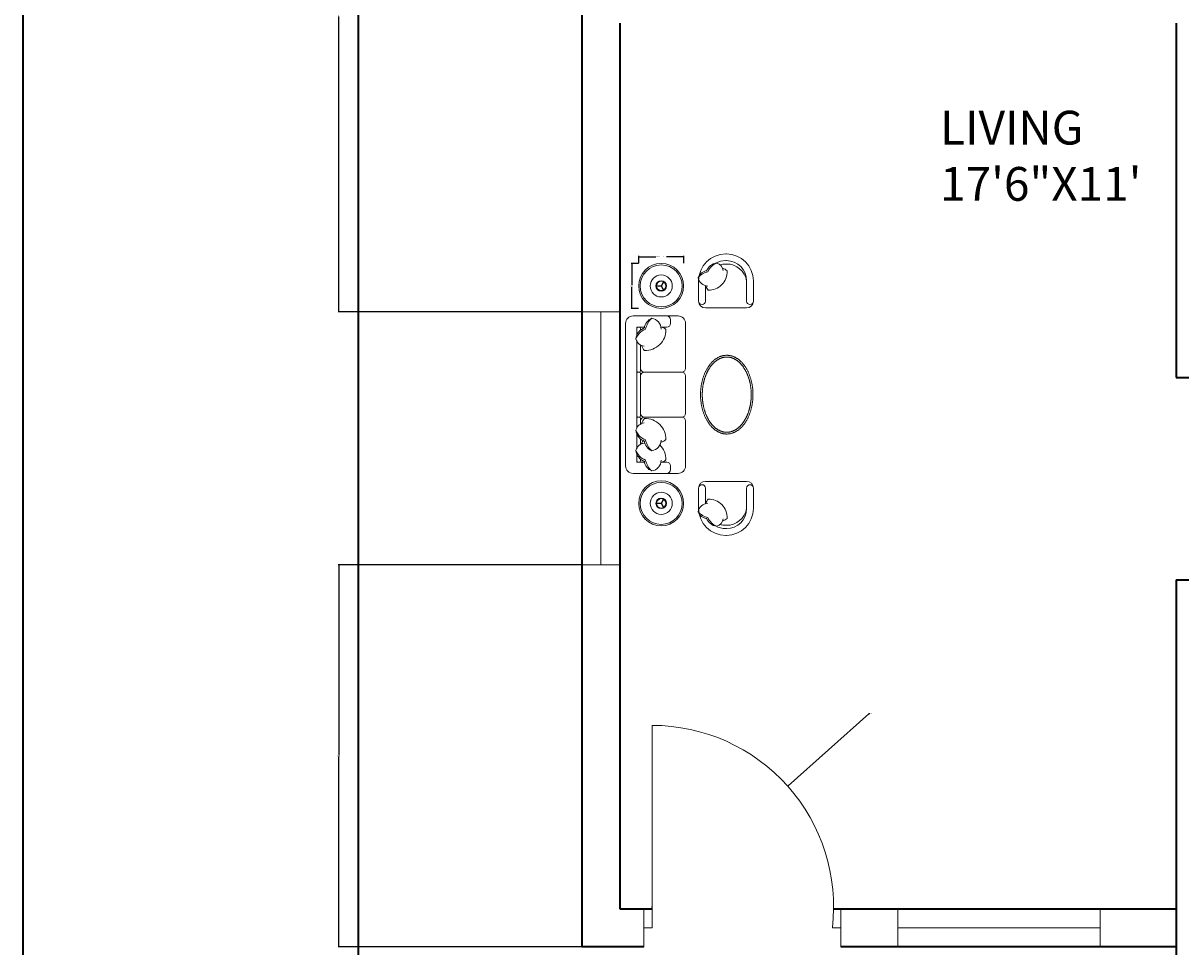
# Model space of a CAD drawing. Units: inches. Extents: x 1976 to 2558, y -977 to 2909.
# Tile 4 of 8: x 1976 to 2251, y 2026 to 2245. Entities that reach past the tile are written whole.
import ezdxf

# ---------------------------------------------------------------- set-up
doc = ezdxf.new("R2010")
doc.units = ezdxf.units.IN
for name, color, linetype, lineweight in [('A-ANNO-DIMS', 2, 'Continuous', 18), ('A-ANNO-TTLB', 7, 'Continuous', 35), ('A-AREA-IDEN', 7, 'Continuous', 18), ('A-DOOR', 3, 'Continuous', 18), ('A-FURN', 8, 'Continuous', 13), ('A-GLAZ', 4, 'Continuous', 18), ('A-WALL', 7, 'Continuous', 35)]:
    doc.layers.add(name, color=color, linetype=linetype, lineweight=lineweight)
doc.styles.get("Standard").update_dxf_attribs({"font": 'arial.ttf'})
doc.dimstyles.get("Standard").update_dxf_attribs({"dimtxt": 0.18, "dimasz": 0.18, "dimexe": 0.18, "dimexo": 0.0625, "dimgap": 0.09, "dimtad": 0, "dimtih": 1, "dimtoh": 1, "dimdec": 4, "dimzin": 0, "dimdsep": 46, "dimtxsty": 'Standard', "dimcen": 0.09, "dimadec": 0, "dimazin": 0, "dimtfac": 1, "dimtdec": 4, "dimtofl": 0, "dimtmove": 0, "dimatfit": 3, "dimfxl": 1, "dimtolj": 1, "dimtzin": 0, "dimarcsym": 0})

# ---------------------------------------------------------------- blocks, each defined once
blk = doc.blocks.new('TABLE-END-ROUND')
at = {"ltscale": 0.03}
for p, q in [((5.29, 5.36), (5.91, 6.45)), ((5.38, 5.31), (6.01, 6.39)), ((5.33, 5.39), (4.08, 5.39)), ((5.33, 5.28), (4.08, 5.28)), ((5.29, 5.31), (5.91, 4.22)), ((5.38, 5.36), (6.01, 4.28))]:
    blk.add_line(p, q, dxfattribs=at)
for radius in [5.33, 2.62, 1.25, 1.12]:
    blk.add_circle((5.33, 5.33), radius, dxfattribs=at)
blk.add_circle((5.33, 5.33), 4.98)
blk = doc.blocks.new('WIN-60-PLAN')
for p, q in [((4.5, 60), (0, 60)), ((0, 60), (9, 60)), ((4.5, 0), (4.5, 60)), ((0, 0), (9, 0)), ((9, 0), (4.5, 0))]:
    blk.add_line(p, q)
blk = doc.blocks.new('*D17')
at = {"layer": 'A-ANNO-DIMS', "color": 0, "lineweight": -2, "transparency": 16777216}
for p, q in [((2121.92, 2188.58), (2121.92, 2190.29)), ((2122.1, 2190.11), (2126, 2190.11)), ((2132.41, 2190.11), (2128.51, 2190.11)), ((2132.59, 2188.58), (2132.59, 2190.29))]:
    blk.add_line(p, q, dxfattribs=at)
at = {"layer": 'A-ANNO-DIMS', "color": 0, "transparency": 16777216}
for points in [[(2122.1, 2190.14), (2122.1, 2190.08), (2121.92, 2190.11)], [(2132.41, 2190.14), (2132.41, 2190.08), (2132.59, 2190.11)]]:
    blk.add_solid(points, dxfattribs=at)
at = {"layer": 'Defpoints', "color": 0, "transparency": 16777216}
for p in [(2132.59, 2190.11), (2121.92, 2188.51), (2132.59, 2188.51)]:
    blk.add_point(p, dxfattribs=at)
at = {"layer": 'A-ANNO-DIMS', "color": 0, "transparency": 16777216, "insert": (2127.26, 2190.11), "char_height": 0.18, "attachment_point": 5}
blk.add_mtext('\\A1;END TABLE 11 TYP.', dxfattribs=at)
blk = doc.blocks.new('*D18')
at = {"layer": 'A-ANNO-DIMS', "color": 0, "lineweight": -2, "transparency": 16777216}
for p, q in [((2121.86, 2188.51), (2120.14, 2188.51)), ((2120.32, 2188.33), (2120.32, 2183.36)), ((2120.32, 2178.03), (2120.32, 2183)), ((2121.86, 2177.85), (2120.14, 2177.85))]:
    blk.add_line(p, q, dxfattribs=at)
at = {"layer": 'A-ANNO-DIMS', "color": 0, "transparency": 16777216}
for points in [[(2120.29, 2188.33), (2120.35, 2188.33), (2120.32, 2188.51)], [(2120.29, 2178.03), (2120.35, 2178.03), (2120.32, 2177.85)]]:
    blk.add_solid(points, dxfattribs=at)
at = {"layer": 'Defpoints', "color": 0, "transparency": 16777216}
for p in [(2120.32, 2188.51), (2121.92, 2188.51), (2121.92, 2177.85)]:
    blk.add_point(p, dxfattribs=at)
at = {"layer": 'A-ANNO-DIMS', "color": 0, "transparency": 16777216, "insert": (2120.32, 2183.18), "char_height": 0.18, "attachment_point": 5}
blk.add_mtext('\\A1;11 TYP.', dxfattribs=at)
blk = doc.blocks.new('*D35')
at = {"layer": 'A-ANNO-DIMS', "color": 0, "lineweight": -2, "transparency": 16777216}
for p, q in [((2108.38, 2317.5), (2050.58, 2317.5)), ((2050.76, 2317.32), (2050.76, 2247.46)), ((2050.76, 2177.24), (2050.76, 2247.1)), ((2108.38, 2177.06), (2050.58, 2177.06))]:
    blk.add_line(p, q, dxfattribs=at)
at = {"layer": 'A-ANNO-DIMS', "color": 0, "transparency": 16777216}
for points in [[(2050.73, 2317.32), (2050.79, 2317.32), (2050.76, 2317.5)], [(2050.73, 2177.24), (2050.79, 2177.24), (2050.76, 2177.06)]]:
    blk.add_solid(points, dxfattribs=at)
at = {"layer": 'Defpoints', "color": 0, "transparency": 16777216}
for p in [(2108.44, 2317.5), (2050.76, 2177.06), (2108.44, 2177.06)]:
    blk.add_point(p, dxfattribs=at)
at = {"layer": 'A-ANNO-DIMS', "color": 0, "transparency": 16777216, "insert": (2050.76, 2247.28), "char_height": 0.18, "attachment_point": 5}
blk.add_mtext('\\A1;140.44', dxfattribs=at)
blk = doc.blocks.new('*D36')
at = {"layer": 'A-ANNO-DIMS', "color": 0, "lineweight": -2, "transparency": 16777216}
for p, q in [((2108.38, 2117.06), (2050.58, 2117.06)), ((2050.76, 2116.88), (2050.76, 2071.95)), ((2050.76, 2026.66), (2050.76, 2071.59)), ((2108.38, 2026.48), (2050.58, 2026.48))]:
    blk.add_line(p, q, dxfattribs=at)
at = {"layer": 'A-ANNO-DIMS', "color": 0, "transparency": 16777216}
for points in [[(2050.73, 2116.88), (2050.79, 2116.88), (2050.76, 2117.06)], [(2050.73, 2026.66), (2050.79, 2026.66), (2050.76, 2026.48)]]:
    blk.add_solid(points, dxfattribs=at)
at = {"layer": 'Defpoints', "color": 0, "transparency": 16777216}
for p in [(2108.44, 2117.06), (2050.76, 2026.48), (2108.44, 2026.48)]:
    blk.add_point(p, dxfattribs=at)
at = {"layer": 'A-ANNO-DIMS', "color": 0, "transparency": 16777216, "insert": (2050.76, 2071.77), "char_height": 0.18, "attachment_point": 5}
blk.add_mtext('\\A1;90.58', dxfattribs=at)
blk = doc.blocks.new('*D88')
at = {"layer": 'A-ANNO-DIMS', "color": 0, "lineweight": -2, "transparency": 16777216}
for p, q in [((2176.55, 2081.75), (2157.4, 2064.69)), ((2176.73, 2081.75), (2176.55, 2081.75)), ((2125.03, 2035.93), (2125.21, 2035.93)), ((2125.12, 2035.84), (2125.12, 2036.02))]:
    blk.add_line(p, q, dxfattribs=at)
at = {"layer": 'A-ANNO-DIMS', "color": 0, "transparency": 16777216}
blk.add_solid([(2157.38, 2064.71), (2157.42, 2064.66), (2157.27, 2064.57)], dxfattribs=at)
at = {"layer": 'Defpoints', "color": 0, "transparency": 16777216}
for p in [(2157.27, 2064.57), (2125.12, 2035.93)]:
    blk.add_point(p, dxfattribs=at)
at = {"layer": 'A-ANNO-DIMS', "color": 0, "transparency": 16777216, "insert": (2177.21, 2081.75), "char_height": 0.18, "attachment_point": 5}
blk.add_mtext('\\A1;R43.05', dxfattribs=at)

msp = doc.modelspace()

# ---------------------------------------------------------------- linework, layer by layer
at = {"layer": 'A-ANNO-TTLB'}
for points in [[(1975.8545, 2909.3429), (2557.9168, 2909.3429), (2557.9168, 1747.8598), (1975.8545, 1747.8598)], [(2055.4343, 2428.9091), (2450.0007, 2428.9091), (2450.0007, 1815.3916), (2055.4343, 1815.3916)]]:
    msp.add_lwpolyline(points, close=True, dxfattribs=at)
at = {"layer": 'A-DOOR'}
for p, q in [((2125.1248, 2030.9789), (2125.1248, 2078.9789)), ((2123.1248, 2035.4789), (2123.1248, 2026.4789)), ((2169.8866, 2035.4789), (2169.8866, 2026.4789)), ((2123.1248, 2026.4789), (2123.1248, 2030.9789)), ((2123.1248, 2030.9789), (2125.1248, 2030.9789)), ((2169.8866, 2030.9789), (2167.8866, 2030.9789)), ((2169.8866, 2026.4789), (2169.8866, 2030.9789))]:
    msp.add_line(p, q, dxfattribs=at)
msp.add_arc((2125.1248, 2035.9313), 43.0476, 353.393764, 90, dxfattribs=at)
at = {"layer": 'A-FURN', "ltscale": 0.03}
for points in [[(2142.6352, 2177.9535), (2147.5242, 2177.9535, 0.41421356), (2149.1272, 2179.5565), (2149.1272, 2184.3654, 0.41421356), (2142.7153, 2190.7772), (2142.6352, 2190.7772), (2142.555, 2190.7772, 0.41421356), (2136.1432, 2184.3654), (2136.1432, 2179.5565, 0.41421356), (2137.7462, 2177.9535), (2142.6352, 2177.9535)], [(2142.6352, 2136.8478), (2147.5242, 2136.8478, -0.41421356), (2149.1272, 2135.2449), (2149.1272, 2130.436, -0.41421356), (2142.7153, 2124.0241), (2142.6352, 2124.0241), (2142.555, 2124.0241, -0.41421356), (2136.1432, 2130.436), (2136.1432, 2135.2449, -0.41421356), (2137.7462, 2136.8478), (2142.6352, 2136.8478)]]:
    msp.add_lwpolyline(points, format="xyb", dxfattribs=at)
at = {"layer": 'A-FURN'}
for points in [[(2136.0121, 2185.1744, -0.14772988), (2138.3546, 2186.5519, -0.21334276), (2140.4215, 2188.5721, -0.17866181)], [(2138.3087, 2183.1542, -0.35677236), (2136.0121, 2185.1744, -0.24954205), (2138.093, 2186.8393, 9.61688035)], [(2137.9047, 2183.2031, 0.16554063), (2138.4005, 2182.1441, 0.42598917), (2142.9018, 2186.7355, 0.12152332), (2141.8333, 2187.3684, -7.11546429)], [(2138.031, 2186.6616, -0.30666349), (2140.4215, 2188.5721, -0.30632997), (2141.9832, 2186.8273, 0.87284716)], [(2140.168, 2188.54, -0.13059149), (2142.555, 2189.1743), (2142.6352, 2189.1743)], [(2141.1886, 2188.2001, -0.07238424), (2142.555, 2188.3728), (2142.6352, 2188.3728)], [(2147.5242, 2184.3654, 0.41421356), (2142.7153, 2189.1743), (2142.6352, 2189.1743)], [(2147.5242, 2184.3654, 0.37271891), (2142.7153, 2188.3728), (2142.6352, 2188.3728)], [(2147.5242, 2184.3654), (2147.5242, 2179.5565, 0.41421356), (2148.3257, 2178.755), (2148.3257, 2178.755, 0.41421356), (2149.1272, 2179.5565)], [(2137.7462, 2183.2416), (2137.7462, 2179.5565, -0.41421356), (2136.9447, 2178.755), (2136.9447, 2178.755, -0.41421356), (2136.1432, 2179.5565)], [(2128.5903, 2176.0679, -0.41421356), (2129.4793, 2175.179), (2129.4793, 2174.2901, -0.41421356), (2128.5903, 2173.4012), (2127.2131, 2173.4012)], [(2125.0263, 2175.5022, 0.14772988), (2123.4986, 2172.9041, 0.21334276), (2121.258, 2170.6117, 0.17866181)], [(2123.3768, 2173.263, 0.30666349), (2121.258, 2170.6117, 0.30632997), (2123.193, 2168.8797, -0.87284716)], [(2122.3679, 2172.7228), (2122.3679, 2173.0456, 0.41421356), (2122.0124, 2173.4012), (2121.8346, 2173.4012, 0.41421356), (2121.479, 2173.0456)], [(2121.479, 2173.0456), (2121.479, 2171.5311, 0.41421356)], [(2127.2127, 2173.4031, -0.16554063), (2128.3872, 2172.8532, -0.42598917), (2123.2949, 2167.8609, -0.12152332), (2122.593, 2169.0459, 7.11546429)], [(2127.2669, 2172.9551, 0.35677236), (2125.0263, 2175.5022, 0.24954205), (2123.1798, 2173.1943, -9.61688035)], [(2121.479, 2170.0523), (2121.479, 2163.0897, 0.41421356), (2121.8346, 2162.7342), (2122.0124, 2162.7342, 0.41421356), (2122.3679, 2163.0897), (2122.3679, 2169.1572, 0.41421356)], [(2122.3679, 2163.6231, 0.41421356), (2123.2568, 2162.7342), (2132.146, 2162.7342, 0.41421356)], [(2122.3679, 2161.8453, -0.41421356), (2123.2568, 2162.7342)], [(2121.479, 2149.5376), (2121.479, 2151.7116, -0.41421356), (2121.8346, 2152.0672), (2122.0124, 2152.0672, -0.41421356), (2122.3679, 2151.7116), (2122.3679, 2150.4327, -0.41421356)], [(2122.3679, 2152.9561, 0.41421356), (2123.2568, 2152.0672)], [(2122.3679, 2151.1783, -0.41421356), (2123.2568, 2152.0672), (2132.146, 2152.0672, -0.41421356)], [(2127.2127, 2146.1868, 0.16554063), (2128.3872, 2146.7367, 0.42598917), (2123.2949, 2151.7291, 0.12152332), (2122.593, 2150.544, -7.11546429)], [(2123.3768, 2146.3269, -0.30666349), (2121.258, 2148.9782, -0.30632997), (2123.193, 2150.7102, 0.87284716)], [(2125.0263, 2144.0878, -0.14772988), (2123.4986, 2146.6858, -0.21334276), (2121.258, 2148.9782, -0.17866181)], [(2123.3768, 2141.5383, -0.30666349), (2121.258, 2144.1896, -0.30632997), (2123.193, 2145.9217, 0.87284716)], [(2121.479, 2144.7491), (2121.479, 2148.0588, -0.41421356)], [(2122.3679, 2146.8671), (2122.3679, 2145.6442, -0.41421356)], [(2122.9405, 2146.5007, 0.07186538), (2122.593, 2145.7554, -7.11546429)], [(2127.2669, 2146.6349, -0.35677236), (2125.0263, 2144.0878, -0.24954205), (2123.1798, 2146.3957, 9.61688035)], [(2125.0263, 2139.2992, -0.14772988), (2123.4986, 2141.8972, -0.21334276), (2121.258, 2144.1896, -0.17866181)], [(2121.479, 2143.2702), (2121.479, 2141.4002), (2123.2259, 2141.4002, -0.41421356)], [(2121.479, 2141.7558), (2121.479, 2143.2702, -0.41421356)], [(2127.2127, 2141.3983, 0.16554063), (2128.3872, 2141.9482, 0.20023115), (2126.9568, 2145.4769, 0.12152332)], [(2122.3679, 2142.0786), (2122.3679, 2141.7558, -0.41421356), (2122.0124, 2141.4002), (2121.8346, 2141.4002, -0.41421356), (2121.479, 2141.7558)], [(2127.2669, 2141.8463, -0.35677236), (2125.0263, 2139.2992, -0.24954205), (2123.1798, 2141.6071, 9.61688035)], [(2127.2131, 2141.4002), (2128.5903, 2141.4002, -0.41421356), (2129.4793, 2140.5113), (2129.4793, 2139.6224, -0.41421356), (2128.5903, 2138.7335)], [(2137.7462, 2131.5597), (2137.7462, 2135.2449, 0.41421356), (2136.9447, 2136.0464), (2136.9447, 2136.0464, 0.41421356), (2136.1432, 2135.2449)], [(2147.5242, 2130.4359), (2147.5242, 2135.2449, -0.41421356), (2148.3257, 2136.0464), (2148.3257, 2136.0464, -0.41421356), (2149.1272, 2135.2449)], [(2137.9047, 2131.5983, -0.16554063), (2138.4005, 2132.6573, -0.42598917), (2142.9018, 2128.0658, -0.12152332), (2141.8333, 2127.433, 7.11546429)], [(2138.3087, 2131.6472, 0.35677236), (2136.0121, 2129.6269, 0.24954205), (2138.093, 2127.9621, -9.61688035)], [(2136.0121, 2129.6269, 0.14772988), (2138.3546, 2128.2495, 0.21334276), (2140.4215, 2126.2293, 0.17866181)], [(2147.5242, 2130.436, -0.37271891), (2142.7153, 2126.4286), (2142.6352, 2126.4286)], [(2147.5242, 2130.436, -0.41421356), (2142.7153, 2125.6271), (2142.6352, 2125.6271)], [(2138.031, 2128.1397, 0.30666349), (2140.4215, 2126.2293, 0.30632997), (2141.9832, 2127.974, -0.87284716)], [(2140.168, 2126.2614, 0.13059149), (2142.555, 2125.6271), (2142.6352, 2125.6271)], [(2141.1886, 2126.6013, 0.07238424), (2142.555, 2126.4286), (2142.6352, 2126.4286)]]:
    msp.add_lwpolyline(points, format="xyb", dxfattribs=at)
at = {"layer": 'A-FURN', "ltscale": 0.03}
msp.add_lwpolyline([(2131.2571, 2176.0679, -0.41421356), (2133.0349, 2174.2901), (2133.0349, 2163.6231, -0.41421356), (2132.146, 2162.7342, -0.41421356), (2133.0349, 2161.8453), (2133.0349, 2152.9561, -0.41421356), (2132.146, 2152.0672, -0.41421356), (2133.0349, 2151.1783), (2133.0349, 2140.5113, -0.41421356), (2131.2571, 2138.7335), (2120.5901, 2138.7335, -0.41421356), (2118.8123, 2140.5113), (2118.8123, 2174.2901, -0.41421356), (2120.5901, 2176.0679)], format="xyb", close=True, dxfattribs=at)
at = {"layer": 'A-FURN'}
for points in [[(2123.2259, 2173.4012), (2121.479, 2173.4012), (2121.479, 2171.5311)], [(2121.479, 2170.0523), (2121.479, 2149.5376)], [(2121.479, 2148.0588), (2121.479, 2144.7491)]]:
    msp.add_lwpolyline(points, dxfattribs=at)
msp.add_lwpolyline([(2121.479, 2152.4228), (2121.479, 2162.3786, -0.41421356), (2121.8346, 2162.7342), (2122.0124, 2162.7342, -0.41421356), (2122.3679, 2162.3786), (2122.3679, 2152.4228, -0.41421356), (2122.0124, 2152.0672), (2121.8346, 2152.0672, -0.41421356)], format="xyb", close=True, dxfattribs=at)
at = {"layer": 'A-FURN', "ltscale": 0.03}
msp.add_polyline3d([(2142.813, 2166.7343, 0), (2142.6952, 2166.7326, 0), (2142.5775, 2166.7276, 0), (2142.4599, 2166.7192, 0), (2142.3424, 2166.7076, 0), (2142.2251, 2166.6925, 0), (2142.1079, 2166.6742, 0), (2141.9911, 2166.6525, 0), (2141.8745, 2166.6275, 0), (2141.7583, 2166.5992, 0), (2141.6424, 2166.5676, 0), (2141.5269, 2166.5328, 0), (2141.412, 2166.4946, 0), (2141.2975, 2166.4532, 0), (2141.1836, 2166.4086, 0), (2141.0702, 2166.3607, 0), (2140.9575, 2166.3096, 0), (2140.8454, 2166.2554, 0), (2140.734, 2166.1979, 0), (2140.6234, 2166.1374, 0), (2140.5136, 2166.0736, 0), (2140.4046, 2166.0068, 0), (2140.2965, 2165.9369, 0), (2140.1892, 2165.8639, 0), (2140.0829, 2165.7879, 0), (2139.9776, 2165.709, 0), (2139.8733, 2165.627, 0), (2139.77, 2165.5421, 0), (2139.6678, 2165.4542, 0), (2139.5668, 2165.3635, 0), (2139.4669, 2165.2699, 0), (2139.3682, 2165.1735, 0), (2139.2708, 2165.0744, 0), (2139.1746, 2164.9724, 0), (2139.0797, 2164.8678, 0), (2138.9862, 2164.7605, 0), (2138.894, 2164.6505, 0), (2138.8033, 2164.538, 0), (2138.714, 2164.4229, 0), (2138.6261, 2164.3053, 0), (2138.5397, 2164.1852, 0), (2138.4549, 2164.0627, 0), (2138.3716, 2163.9378, 0), (2138.29, 2163.8105, 0), (2138.2099, 2163.681, 0), (2138.1315, 2163.5492, 0), (2138.0548, 2163.4152, 0), (2137.9797, 2163.2791, 0), (2137.9064, 2163.1408, 0), (2137.8349, 2163.0005, 0), (2137.7651, 2162.8582, 0), (2137.6972, 2162.7139, 0), (2137.6311, 2162.5678, 0), (2137.5668, 2162.4198, 0), (2137.5044, 2162.2699, 0), (2137.444, 2162.1184, 0), (2137.3854, 2161.9651, 0), (2137.3288, 2161.8102, 0), (2137.2741, 2161.6538, 0), (2137.2215, 2161.4958, 0), (2137.1708, 2161.3363, 0), (2137.1222, 2161.1755, 0), (2137.0756, 2161.0133, 0), (2137.031, 2160.8497, 0), (2136.9885, 2160.685, 0), (2136.9481, 2160.5191, 0), (2136.9098, 2160.352, 0), (2136.8737, 2160.1839, 0), (2136.8396, 2160.0148, 0), (2136.8077, 2159.8448, 0), (2136.7779, 2159.6739, 0), (2136.7503, 2159.5022, 0), (2136.7249, 2159.3297, 0), (2136.7017, 2159.1566, 0), (2136.6806, 2158.9828, 0), (2136.6618, 2158.8084, 0), (2136.6451, 2158.6336, 0), (2136.6306, 2158.4582, 0), (2136.6184, 2158.2826, 0), (2136.6084, 2158.1066, 0), (2136.6006, 2157.9303, 0), (2136.595, 2157.7539, 0), (2136.5917, 2157.5773, 0), (2136.5906, 2157.4007, 0), (2136.5917, 2157.224, 0), (2136.595, 2157.0475, 0), (2136.6006, 2156.871, 0), (2136.6084, 2156.6948, 0), (2136.6184, 2156.5188, 0), (2136.6306, 2156.3431, 0), (2136.6451, 2156.1678, 0), (2136.6618, 2155.9929, 0), (2136.6806, 2155.8186, 0), (2136.7017, 2155.6448, 0), (2136.7249, 2155.4716, 0), (2136.7503, 2155.2992, 0), (2136.7779, 2155.1274, 0), (2136.8077, 2154.9565, 0), (2136.8396, 2154.7865, 0), (2136.8737, 2154.6174, 0), (2136.9098, 2154.4493, 0), (2136.9481, 2154.2823, 0), (2136.9885, 2154.1164, 0), (2137.031, 2153.9516, 0), (2137.0756, 2153.7881, 0), (2137.1222, 2153.6259, 0), (2137.1708, 2153.465, 0), (2137.2215, 2153.3056, 0), (2137.2741, 2153.1476, 0), (2137.3288, 2152.9911, 0), (2137.3854, 2152.8362, 0), (2137.444, 2152.683, 0), (2137.5044, 2152.5314, 0), (2137.5668, 2152.3816, 0), (2137.6311, 2152.2336, 0), (2137.6972, 2152.0874, 0), (2137.7651, 2151.9431, 0), (2137.8349, 2151.8008, 0), (2137.9064, 2151.6605, 0), (2137.9797, 2151.5223, 0), (2138.0548, 2151.3861, 0), (2138.1315, 2151.2521, 0), (2138.2099, 2151.1204, 0), (2138.29, 2150.9908, 0), (2138.3716, 2150.8636, 0), (2138.4549, 2150.7387, 0), (2138.5397, 2150.6161, 0), (2138.6261, 2150.4961, 0), (2138.714, 2150.3785, 0), (2138.8033, 2150.2634, 0), (2138.894, 2150.1508, 0), (2138.9862, 2150.0409, 0), (2139.0797, 2149.9336, 0), (2139.1746, 2149.8289, 0), (2139.2708, 2149.727, 0), (2139.3682, 2149.6278, 0), (2139.4669, 2149.5314, 0), (2139.5668, 2149.4379, 0), (2139.6678, 2149.3471, 0), (2139.77, 2149.2593, 0), (2139.8733, 2149.1744, 0), (2139.9776, 2149.0924, 0), (2140.0829, 2149.0134, 0), (2140.1892, 2148.9374, 0), (2140.2965, 2148.8645, 0), (2140.4046, 2148.7945, 0), (2140.5136, 2148.7277, 0), (2140.6234, 2148.664, 0), (2140.734, 2148.6034, 0), (2140.8454, 2148.546, 0), (2140.9575, 2148.4917, 0), (2141.0702, 2148.4406, 0), (2141.1836, 2148.3928, 0), (2141.2975, 2148.3481, 0), (2141.412, 2148.3067, 0), (2141.5269, 2148.2686, 0), (2141.6424, 2148.2337, 0), (2141.7583, 2148.2021, 0), (2141.8745, 2148.1738, 0), (2141.9911, 2148.1489, 0), (2142.1079, 2148.1272, 0), (2142.2251, 2148.1088, 0), (2142.3424, 2148.0938, 0), (2142.4599, 2148.0821, 0), (2142.5775, 2148.0738, 0), (2142.6952, 2148.0687, 0), (2142.813, 2148.0671, 0), (2142.9307, 2148.0687, 0), (2143.0484, 2148.0738, 0), (2143.1661, 2148.0821, 0), (2143.2836, 2148.0938, 0), (2143.4009, 2148.1088, 0), (2143.518, 2148.1272, 0), (2143.6349, 2148.1489, 0), (2143.7515, 2148.1738, 0), (2143.8677, 2148.2021, 0), (2143.9836, 2148.2337, 0), (2144.099, 2148.2686, 0), (2144.214, 2148.3067, 0), (2144.3285, 2148.3481, 0), (2144.4424, 2148.3928, 0), (2144.5558, 2148.4406, 0), (2144.6685, 2148.4917, 0), (2144.7806, 2148.546, 0), (2144.8919, 2148.6034, 0), (2145.0025, 2148.664, 0), (2145.1124, 2148.7277, 0), (2145.2214, 2148.7945, 0), (2145.3295, 2148.8645, 0), (2145.4368, 2148.9374, 0), (2145.5431, 2149.0134, 0), (2145.6484, 2149.0924, 0), (2145.7527, 2149.1744, 0), (2145.8559, 2149.2593, 0), (2145.9581, 2149.3471, 0), (2146.0592, 2149.4379, 0), (2146.159, 2149.5314, 0), (2146.2577, 2149.6278, 0), (2146.3552, 2149.727, 0), (2146.4513, 2149.8289, 0), (2146.5462, 2149.9336, 0), (2146.6397, 2150.0409, 0), (2146.7319, 2150.1508, 0), (2146.8227, 2150.2634, 0), (2146.912, 2150.3785, 0), (2146.9999, 2150.4961, 0), (2147.0862, 2150.6161, 0), (2147.1711, 2150.7387, 0), (2147.2543, 2150.8636, 0), (2147.336, 2150.9908, 0), (2147.4161, 2151.1204, 0), (2147.4945, 2151.2521, 0), (2147.5712, 2151.3861, 0), (2147.6462, 2151.5223, 0), (2147.7195, 2151.6605, 0), (2147.7911, 2151.8008, 0), (2147.8608, 2151.9431, 0), (2147.9288, 2152.0874, 0), (2147.9949, 2152.2336, 0), (2148.0591, 2152.3816, 0), (2148.1215, 2152.5314, 0), (2148.182, 2152.683, 0), (2148.2406, 2152.8362, 0), (2148.2972, 2152.9911, 0), (2148.3518, 2153.1476, 0), (2148.4045, 2153.3056, 0), (2148.4552, 2153.465, 0), (2148.5038, 2153.6259, 0), (2148.5504, 2153.7881, 0), (2148.595, 2153.9516, 0), (2148.6374, 2154.1164, 0), (2148.6778, 2154.2823, 0), (2148.7161, 2154.4493, 0), (2148.7523, 2154.6174, 0), (2148.7863, 2154.7865, 0), (2148.8183, 2154.9565, 0), (2148.848, 2155.1274, 0), (2148.8756, 2155.2992, 0), (2148.901, 2155.4716, 0), (2148.9243, 2155.6448, 0), (2148.9453, 2155.8186, 0), (2148.9642, 2155.9929, 0), (2148.9809, 2156.1678, 0), (2148.9953, 2156.3431, 0), (2149.0075, 2156.5188, 0), (2149.0176, 2156.6948, 0), (2149.0254, 2156.871, 0), (2149.0309, 2157.0475, 0), (2149.0343, 2157.224, 0), (2149.0354, 2157.4007, 0), (2149.0343, 2157.5773, 0), (2149.0309, 2157.7539, 0), (2149.0254, 2157.9303, 0), (2149.0176, 2158.1066, 0), (2149.0075, 2158.2826, 0), (2148.9953, 2158.4582, 0), (2148.9809, 2158.6336, 0), (2148.9642, 2158.8084, 0), (2148.9453, 2158.9828, 0), (2148.9243, 2159.1566, 0), (2148.901, 2159.3297, 0), (2148.8756, 2159.5022, 0), (2148.848, 2159.6739, 0), (2148.8183, 2159.8448, 0), (2148.7863, 2160.0148, 0), (2148.7523, 2160.1839, 0), (2148.7161, 2160.352, 0), (2148.6778, 2160.5191, 0), (2148.6374, 2160.685, 0), (2148.595, 2160.8497, 0), (2148.5504, 2161.0133, 0), (2148.5038, 2161.1755, 0), (2148.4552, 2161.3363, 0), (2148.4045, 2161.4958, 0), (2148.3518, 2161.6538, 0), (2148.2972, 2161.8102, 0), (2148.2406, 2161.9651, 0), (2148.182, 2162.1184, 0), (2148.1215, 2162.2699, 0), (2148.0591, 2162.4198, 0), (2147.9949, 2162.5678, 0), (2147.9288, 2162.7139, 0), (2147.8608, 2162.8582, 0), (2147.7911, 2163.0005, 0), (2147.7195, 2163.1408, 0), (2147.6462, 2163.2791, 0), (2147.5712, 2163.4152, 0), (2147.4945, 2163.5492, 0), (2147.4161, 2163.681, 0), (2147.336, 2163.8105, 0), (2147.2543, 2163.9378, 0), (2147.1711, 2164.0627, 0), (2147.0862, 2164.1852, 0), (2146.9999, 2164.3053, 0), (2146.912, 2164.4229, 0), (2146.8227, 2164.538, 0), (2146.7319, 2164.6505, 0), (2146.6397, 2164.7605, 0), (2146.5462, 2164.8678, 0), (2146.4513, 2164.9724, 0), (2146.3552, 2165.0744, 0), (2146.2577, 2165.1735, 0), (2146.159, 2165.2699, 0), (2146.0592, 2165.3635, 0), (2145.9581, 2165.4542, 0), (2145.8559, 2165.5421, 0), (2145.7527, 2165.627, 0), (2145.6484, 2165.709, 0), (2145.5431, 2165.7879, 0), (2145.4368, 2165.8639, 0), (2145.3295, 2165.9369, 0), (2145.2214, 2166.0068, 0), (2145.1124, 2166.0736, 0), (2145.0025, 2166.1374, 0), (2144.8919, 2166.1979, 0), (2144.7806, 2166.2554, 0), (2144.6685, 2166.3096, 0), (2144.5558, 2166.3607, 0), (2144.4424, 2166.4086, 0), (2144.3285, 2166.4532, 0), (2144.214, 2166.4946, 0), (2144.099, 2166.5328, 0), (2143.9836, 2166.5676, 0), (2143.8677, 2166.5992, 0), (2143.7515, 2166.6275, 0), (2143.6349, 2166.6525, 0), (2143.518, 2166.6742, 0), (2143.4009, 2166.6925, 0), (2143.2836, 2166.7076, 0), (2143.1661, 2166.7192, 0), (2143.0484, 2166.7276, 0), (2142.9307, 2166.7326, 0), (2142.813, 2166.7343, 0)], dxfattribs=at)
at = {"layer": 'A-FURN'}
msp.add_polyline3d([(2142.813, 2166.3195, 0), (2142.7493, 2166.3189, 0), (2142.6854, 2166.3173, 0), (2142.6212, 2166.3145, 0), (2142.5567, 2166.3106, 0), (2142.4919, 2166.3056, 0), (2142.4269, 2166.2995, 0), (2142.3617, 2166.2921, 0), (2142.2962, 2166.2836, 0), (2142.2304, 2166.2739, 0), (2142.1645, 2166.2629, 0), (2142.0983, 2166.2508, 0), (2142.0319, 2166.2374, 0), (2141.9653, 2166.2227, 0), (2141.8986, 2166.2068, 0), (2141.8316, 2166.1896, 0), (2141.7645, 2166.1711, 0), (2141.6973, 2166.1513, 0), (2141.6298, 2166.1301, 0), (2141.5623, 2166.1077, 0), (2141.4946, 2166.0838, 0), (2141.4268, 2166.0586, 0), (2141.3588, 2166.032, 0), (2141.2908, 2166.004, 0), (2141.2227, 2165.9745, 0), (2141.1546, 2165.9437, 0), (2141.0865, 2165.9114, 0), (2141.0183, 2165.8778, 0), (2140.9502, 2165.8427, 0), (2140.8821, 2165.8062, 0), (2140.8141, 2165.7682, 0), (2140.7461, 2165.7289, 0), (2140.6783, 2165.6881, 0), (2140.6105, 2165.6459, 0), (2140.5429, 2165.6023, 0), (2140.4755, 2165.5572, 0), (2140.4083, 2165.5107, 0), (2140.3412, 2165.4627, 0), (2140.2744, 2165.4133, 0), (2140.2078, 2165.3625, 0), (2140.1414, 2165.3102, 0), (2140.0754, 2165.2565, 0), (2140.0096, 2165.2014, 0), (2139.9442, 2165.1446, 0), (2139.879, 2165.0864, 0), (2139.8143, 2165.0266, 0), (2139.7499, 2164.9653, 0), (2139.6859, 2164.9025, 0), (2139.6223, 2164.8383, 0), (2139.5591, 2164.7726, 0), (2139.4963, 2164.7055, 0), (2139.434, 2164.637, 0), (2139.3722, 2164.5671, 0), (2139.3108, 2164.4958, 0), (2139.25, 2164.4233, 0), (2139.1896, 2164.3494, 0), (2139.1299, 2164.2742, 0), (2139.0706, 2164.1978, 0), (2139.0119, 2164.1201, 0), (2138.9539, 2164.0412, 0), (2138.8964, 2163.9611, 0), (2138.8395, 2163.8799, 0), (2138.7833, 2163.7974, 0), (2138.7277, 2163.7138, 0), (2138.6729, 2163.6291, 0), (2138.6187, 2163.5434, 0), (2138.5652, 2163.4565, 0), (2138.5124, 2163.3686, 0), (2138.4604, 2163.2797, 0), (2138.4091, 2163.1897, 0), (2138.3586, 2163.0988, 0), (2138.3089, 2163.0069, 0), (2138.26, 2162.9141, 0), (2138.2119, 2162.8203, 0), (2138.1647, 2162.7257, 0), (2138.1183, 2162.6301, 0), (2138.0728, 2162.5338, 0), (2138.0282, 2162.4365, 0), (2137.9845, 2162.3385, 0), (2137.9418, 2162.2397, 0), (2137.9, 2162.1401, 0), (2137.8591, 2162.0398, 0), (2137.8193, 2161.9387, 0), (2137.7804, 2161.837, 0), (2137.7425, 2161.7347, 0), (2137.7056, 2161.6321, 0), (2137.6698, 2161.5292, 0), (2137.6349, 2161.4261, 0), (2137.601, 2161.3226, 0), (2137.5681, 2161.219, 0), (2137.5362, 2161.115, 0), (2137.5053, 2161.0109, 0), (2137.4754, 2160.9065, 0), (2137.4464, 2160.8018, 0), (2137.4184, 2160.697, 0), (2137.3913, 2160.5919, 0), (2137.3652, 2160.4866, 0), (2137.3401, 2160.3811, 0), (2137.3159, 2160.2754, 0), (2137.2926, 2160.1695, 0), (2137.2703, 2160.0635, 0), (2137.2489, 2159.9572, 0), (2137.2285, 2159.8508, 0), (2137.209, 2159.7443, 0), (2137.1904, 2159.6376, 0), (2137.1727, 2159.5307, 0), (2137.1559, 2159.4237, 0), (2137.1401, 2159.3166, 0), (2137.1251, 2159.2093, 0), (2137.1111, 2159.1019, 0), (2137.0979, 2158.9944, 0), (2137.0857, 2158.8868, 0), (2137.0743, 2158.7792, 0), (2137.0638, 2158.6714, 0), (2137.0542, 2158.5635, 0), (2137.0455, 2158.4556, 0), (2137.0376, 2158.3476, 0), (2137.0306, 2158.2395, 0), (2137.0245, 2158.1314, 0), (2137.0192, 2158.0232, 0), (2137.0148, 2157.915, 0), (2137.0113, 2157.8068, 0), (2137.0086, 2157.6985, 0), (2137.0067, 2157.5902, 0), (2137.0056, 2157.4819, 0), (2137.0054, 2157.3736, 0), (2137.006, 2157.2653, 0), (2137.0075, 2157.157, 0), (2137.0098, 2157.0487, 0), (2137.0129, 2156.9405, 0), (2137.0169, 2156.8322, 0), (2137.0218, 2156.724, 0), (2137.0275, 2156.6159, 0), (2137.034, 2156.5078, 0), (2137.0415, 2156.3998, 0), (2137.0497, 2156.2918, 0), (2137.0589, 2156.1839, 0), (2137.0689, 2156.0761, 0), (2137.0799, 2155.9683, 0), (2137.0917, 2155.8607, 0), (2137.1044, 2155.7532, 0), (2137.118, 2155.6457, 0), (2137.1325, 2155.5384, 0), (2137.1479, 2155.4312, 0), (2137.1642, 2155.3241, 0), (2137.1814, 2155.2172, 0), (2137.1995, 2155.1104, 0), (2137.2186, 2155.0038, 0), (2137.2386, 2154.8973, 0), (2137.2595, 2154.791, 0), (2137.2813, 2154.6848, 0), (2137.3041, 2154.5789, 0), (2137.3278, 2154.4731, 0), (2137.3525, 2154.3675, 0), (2137.3781, 2154.2621, 0), (2137.4047, 2154.1569, 0), (2137.4322, 2154.0519, 0), (2137.4607, 2153.9472, 0), (2137.4902, 2153.8427, 0), (2137.5207, 2153.7384, 0), (2137.5521, 2153.6343, 0), (2137.5845, 2153.5305, 0), (2137.6178, 2153.427, 0), (2137.6522, 2153.3237, 0), (2137.6876, 2153.2207, 0), (2137.7239, 2153.1179, 0), (2137.7613, 2153.0155, 0), (2137.7997, 2152.9134, 0), (2137.8391, 2152.812, 0), (2137.8794, 2152.7113, 0), (2137.9208, 2152.6113, 0), (2137.9631, 2152.5121, 0), (2138.0063, 2152.4137, 0), (2138.0504, 2152.3161, 0), (2138.0955, 2152.2193, 0), (2138.1414, 2152.1233, 0), (2138.1882, 2152.0283, 0), (2138.2358, 2151.9341, 0), (2138.2843, 2151.8408, 0), (2138.3336, 2151.7484, 0), (2138.3837, 2151.657, 0), (2138.4346, 2151.5665, 0), (2138.4863, 2151.4771, 0), (2138.5387, 2151.3887, 0), (2138.5918, 2151.3013, 0), (2138.6457, 2151.215, 0), (2138.7002, 2151.1297, 0), (2138.7554, 2151.0456, 0), (2138.8113, 2150.9626, 0), (2138.8679, 2150.8807, 0), (2138.925, 2150.8, 0), (2138.9828, 2150.7205, 0), (2139.0412, 2150.6422, 0), (2139.1002, 2150.5652, 0), (2139.1597, 2150.4894, 0), (2139.2197, 2150.4149, 0), (2139.2803, 2150.3416, 0), (2139.3414, 2150.2697, 0), (2139.403, 2150.1992, 0), (2139.4651, 2150.13, 0), (2139.5276, 2150.0622, 0), (2139.5906, 2149.9958, 0), (2139.654, 2149.9308, 0), (2139.7178, 2149.8673, 0), (2139.782, 2149.8052, 0), (2139.8466, 2149.7447, 0), (2139.9116, 2149.6857, 0), (2139.9768, 2149.6282, 0), (2140.0424, 2149.5722, 0), (2140.1083, 2149.5178, 0), (2140.1746, 2149.4648, 0), (2140.241, 2149.4132, 0), (2140.3077, 2149.3631, 0), (2140.3747, 2149.3145, 0), (2140.4419, 2149.2673, 0), (2140.5092, 2149.2215, 0), (2140.5767, 2149.1771, 0), (2140.6444, 2149.1342, 0), (2140.7122, 2149.0927, 0), (2140.7801, 2149.0526, 0), (2140.8481, 2149.014, 0), (2140.9162, 2148.9768, 0), (2140.9843, 2148.941, 0), (2141.0524, 2148.9066, 0), (2141.1206, 2148.8736, 0), (2141.1887, 2148.8421, 0), (2141.2568, 2148.8119, 0), (2141.3248, 2148.7832, 0), (2141.3928, 2148.7559, 0), (2141.4607, 2148.73, 0), (2141.5284, 2148.7055, 0), (2141.5961, 2148.6823, 0), (2141.6636, 2148.6605, 0), (2141.7309, 2148.64, 0), (2141.7981, 2148.6208, 0), (2141.8651, 2148.603, 0), (2141.932, 2148.5864, 0), (2141.9986, 2148.5711, 0), (2142.0651, 2148.5571, 0), (2142.1314, 2148.5443, 0), (2142.1975, 2148.5328, 0), (2142.2633, 2148.5225, 0), (2142.3289, 2148.5133, 0), (2142.3943, 2148.5054, 0), (2142.4595, 2148.4987, 0), (2142.5244, 2148.4931, 0), (2142.589, 2148.4886, 0), (2142.6533, 2148.4853, 0), (2142.7174, 2148.4831, 0), (2142.7812, 2148.482, 0), (2142.8448, 2148.482, 0), (2142.9085, 2148.4831, 0), (2142.9726, 2148.4853, 0), (2143.037, 2148.4886, 0), (2143.1016, 2148.4931, 0), (2143.1665, 2148.4987, 0), (2143.2316, 2148.5054, 0), (2143.297, 2148.5133, 0), (2143.3626, 2148.5225, 0), (2143.4285, 2148.5328, 0), (2143.4946, 2148.5443, 0), (2143.5608, 2148.5571, 0), (2143.6273, 2148.5711, 0), (2143.694, 2148.5864, 0), (2143.7608, 2148.603, 0), (2143.8279, 2148.6208, 0), (2143.8951, 2148.64, 0), (2143.9624, 2148.6605, 0), (2144.0299, 2148.6823, 0), (2144.0975, 2148.7055, 0), (2144.1653, 2148.73, 0), (2144.2332, 2148.7559, 0), (2144.3011, 2148.7832, 0), (2144.3692, 2148.8119, 0), (2144.4373, 2148.8421, 0), (2144.5054, 2148.8736, 0), (2144.5735, 2148.9066, 0), (2144.6417, 2148.941, 0), (2144.7098, 2148.9768, 0), (2144.7779, 2149.014, 0), (2144.8459, 2149.0526, 0), (2144.9138, 2149.0927, 0), (2144.9816, 2149.1342, 0), (2145.0492, 2149.1771, 0), (2145.1167, 2149.2215, 0), (2145.1841, 2149.2673, 0), (2145.2513, 2149.3145, 0), (2145.3182, 2149.3631, 0), (2145.3849, 2149.4132, 0), (2145.4514, 2149.4648, 0), (2145.5176, 2149.5178, 0), (2145.5835, 2149.5722, 0), (2145.6491, 2149.6282, 0), (2145.7144, 2149.6857, 0), (2145.7793, 2149.7447, 0), (2145.8439, 2149.8052, 0), (2145.9081, 2149.8673, 0), (2145.9719, 2149.9308, 0), (2146.0353, 2149.9958, 0), (2146.0983, 2150.0622, 0), (2146.1608, 2150.13, 0), (2146.2229, 2150.1992, 0), (2146.2845, 2150.2697, 0), (2146.3456, 2150.3416, 0), (2146.4062, 2150.4149, 0), (2146.4663, 2150.4894, 0), (2146.5258, 2150.5652, 0), (2146.5848, 2150.6422, 0), (2146.6431, 2150.7205, 0), (2146.7009, 2150.8, 0), (2146.7581, 2150.8807, 0), (2146.8146, 2150.9626, 0), (2146.8705, 2151.0456, 0), (2146.9257, 2151.1297, 0), (2146.9803, 2151.215, 0), (2147.0341, 2151.3013, 0), (2147.0873, 2151.3887, 0), (2147.1397, 2151.4771, 0), (2147.1913, 2151.5665, 0), (2147.2422, 2151.657, 0), (2147.2923, 2151.7484, 0), (2147.3416, 2151.8408, 0), (2147.3901, 2151.9341, 0), (2147.4378, 2152.0283, 0), (2147.4846, 2152.1233, 0), (2147.5305, 2152.2193, 0), (2147.5755, 2152.3161, 0), (2147.6197, 2152.4137, 0), (2147.6629, 2152.5121, 0), (2147.7052, 2152.6113, 0), (2147.7465, 2152.7113, 0), (2147.7869, 2152.812, 0), (2147.8263, 2152.9134, 0), (2147.8646, 2153.0155, 0), (2147.902, 2153.1179, 0), (2147.9384, 2153.2207, 0), (2147.9737, 2153.3237, 0), (2148.0081, 2153.427, 0), (2148.0415, 2153.5305, 0), (2148.0739, 2153.6343, 0), (2148.1053, 2153.7384, 0), (2148.1357, 2153.8427, 0), (2148.1652, 2153.9472, 0), (2148.1937, 2154.0519, 0), (2148.2212, 2154.1569, 0), (2148.2478, 2154.2621, 0), (2148.2734, 2154.3675, 0), (2148.2981, 2154.4731, 0), (2148.3218, 2154.5789, 0), (2148.3446, 2154.6848, 0), (2148.3665, 2154.791, 0), (2148.3874, 2154.8973, 0), (2148.4074, 2155.0038, 0), (2148.4264, 2155.1104, 0), (2148.4446, 2155.2172, 0), (2148.4618, 2155.3241, 0), (2148.4781, 2155.4312, 0), (2148.4935, 2155.5384, 0), (2148.508, 2155.6457, 0), (2148.5216, 2155.7532, 0), (2148.5343, 2155.8607, 0), (2148.5461, 2155.9683, 0), (2148.557, 2156.0761, 0), (2148.5671, 2156.1839, 0), (2148.5762, 2156.2918, 0), (2148.5845, 2156.3998, 0), (2148.5919, 2156.5078, 0), (2148.5985, 2156.6159, 0), (2148.6042, 2156.724, 0), (2148.609, 2156.8322, 0), (2148.613, 2156.9405, 0), (2148.6162, 2157.0487, 0), (2148.6184, 2157.157, 0), (2148.6199, 2157.2653, 0), (2148.6205, 2157.3736, 0), (2148.6203, 2157.4819, 0), (2148.6193, 2157.5902, 0), (2148.6174, 2157.6985, 0), (2148.6147, 2157.8068, 0), (2148.6111, 2157.915, 0), (2148.6067, 2158.0232, 0), (2148.6014, 2158.1314, 0), (2148.5953, 2158.2395, 0), (2148.5883, 2158.3476, 0), (2148.5805, 2158.4556, 0), (2148.5717, 2158.5635, 0), (2148.5621, 2158.6714, 0), (2148.5517, 2158.7792, 0), (2148.5403, 2158.8868, 0), (2148.528, 2158.9944, 0), (2148.5149, 2159.1019, 0), (2148.5008, 2159.2093, 0), (2148.4859, 2159.3166, 0), (2148.47, 2159.4237, 0), (2148.4533, 2159.5307, 0), (2148.4356, 2159.6376, 0), (2148.417, 2159.7443, 0), (2148.3975, 2159.8508, 0), (2148.377, 2159.9572, 0), (2148.3557, 2160.0635, 0), (2148.3334, 2160.1695, 0), (2148.3101, 2160.2754, 0), (2148.2859, 2160.3811, 0), (2148.2608, 2160.4866, 0), (2148.2347, 2160.5919, 0), (2148.2076, 2160.697, 0), (2148.1796, 2160.8018, 0), (2148.1506, 2160.9065, 0), (2148.1206, 2161.0109, 0), (2148.0897, 2161.115, 0), (2148.0578, 2161.219, 0), (2148.0249, 2161.3226, 0), (2147.991, 2161.4261, 0), (2147.9562, 2161.5292, 0), (2147.9203, 2161.6321, 0), (2147.8835, 2161.7347, 0), (2147.8456, 2161.837, 0), (2147.8067, 2161.9387, 0), (2147.7668, 2162.0398, 0), (2147.726, 2162.1401, 0), (2147.6842, 2162.2397, 0), (2147.6414, 2162.3385, 0), (2147.5977, 2162.4365, 0), (2147.5531, 2162.5338, 0), (2147.5076, 2162.6301, 0), (2147.4613, 2162.7257, 0), (2147.414, 2162.8203, 0), (2147.366, 2162.9141, 0), (2147.3171, 2163.0069, 0), (2147.2674, 2163.0988, 0), (2147.2169, 2163.1897, 0), (2147.1656, 2163.2797, 0), (2147.1136, 2163.3686, 0), (2147.0608, 2163.4565, 0), (2147.0073, 2163.5434, 0), (2146.9531, 2163.6291, 0), (2146.8982, 2163.7138, 0), (2146.8427, 2163.7974, 0), (2146.7864, 2163.8799, 0), (2146.7296, 2163.9611, 0), (2146.6721, 2164.0412, 0), (2146.614, 2164.1201, 0), (2146.5553, 2164.1978, 0), (2146.4961, 2164.2742, 0), (2146.4363, 2164.3494, 0), (2146.376, 2164.4233, 0), (2146.3151, 2164.4958, 0), (2146.2538, 2164.5671, 0), (2146.1919, 2164.637, 0), (2146.1296, 2164.7055, 0), (2146.0669, 2164.7726, 0), (2146.0037, 2164.8383, 0), (2145.9401, 2164.9025, 0), (2145.8761, 2164.9653, 0), (2145.8117, 2165.0266, 0), (2145.7469, 2165.0864, 0), (2145.6818, 2165.1446, 0), (2145.6164, 2165.2014, 0), (2145.5506, 2165.2565, 0), (2145.4845, 2165.3102, 0), (2145.4182, 2165.3625, 0), (2145.3516, 2165.4133, 0), (2145.2848, 2165.4627, 0), (2145.2177, 2165.5107, 0), (2145.1504, 2165.5572, 0), (2145.083, 2165.6023, 0), (2145.0154, 2165.6459, 0), (2144.9477, 2165.6881, 0), (2144.8798, 2165.7289, 0), (2144.8119, 2165.7682, 0), (2144.7438, 2165.8062, 0), (2144.6757, 2165.8427, 0), (2144.6076, 2165.8778, 0), (2144.5395, 2165.9114, 0), (2144.4713, 2165.9437, 0), (2144.4032, 2165.9745, 0), (2144.3351, 2166.004, 0), (2144.2671, 2166.032, 0), (2144.1992, 2166.0586, 0), (2144.1314, 2166.0838, 0), (2144.0637, 2166.1077, 0), (2143.9961, 2166.1301, 0), (2143.9287, 2166.1513, 0), (2143.8614, 2166.1711, 0), (2143.7943, 2166.1896, 0), (2143.7274, 2166.2068, 0), (2143.6606, 2166.2227, 0), (2143.5941, 2166.2374, 0), (2143.5277, 2166.2508, 0), (2143.4615, 2166.2629, 0), (2143.3955, 2166.2739, 0), (2143.3298, 2166.2836, 0), (2143.2643, 2166.2921, 0), (2143.199, 2166.2995, 0), (2143.134, 2166.3056, 0), (2143.0692, 2166.3106, 0), (2143.0048, 2166.3145, 0), (2142.9405, 2166.3173, 0), (2142.8766, 2166.3189, 0), (2142.813, 2166.3195, 0)], dxfattribs=at)
at = {"layer": 'A-GLAZ'}
for p, q in [((2183.4385, 2035.4789), (2183.4385, 2026.4789)), ((2231.4385, 2030.9789), (2231.4385, 2035.4789)), ((2231.4385, 2035.4789), (2231.4385, 2026.4789)), ((2183.4385, 2026.4789), (2183.4385, 2030.9789)), ((2183.4385, 2030.9789), (2231.4385, 2030.9789))]:
    msp.add_line(p, q, dxfattribs=at)
at = {"layer": 'A-WALL'}
for p, q in [((2108.4385, 2317.4977), (2108.4385, 2026.4789)), ((2117.4385, 2245.4789), (2117.4385, 2035.4789)), ((2117.4385, 2245.4789), (2117.4385, 2035.4789)), ((2249.4385, 2245.4789), (2249.4385, 2161.4789)), ((2249.4385, 2161.4789), (2260.6343, 2161.4789)), ((2249.4385, 2113.4789), (2260.6343, 2113.4789)), ((2249.4385, 2113.4789), (2249.4385, 1967.9789)), ((2117.4385, 2035.4789), (2125.1248, 2035.4789)), ((2168.17, 2035.4789), (2249.4385, 2035.4789)), ((2249.4385, 2035.4789), (2249.4385, 2026.4789)), ((2123.1248, 2026.4789), (2108.4385, 2026.4789)), ((2249.4385, 2026.4789), (2169.8866, 2026.4789))]:
    msp.add_line(p, q, dxfattribs=at)

# ---------------------------------------------------------------- block references
at = {"layer": 'A-FURN'}
msp.add_blockref('TABLE-END-ROUND', (2121.923, 2177.846), dxfattribs=at)
at = {"layer": 'A-FURN', "rotation": 239.9999999969837}
msp.add_blockref('TABLE-END-ROUND', (2125.3052, 2138.9081), dxfattribs=at)
at = {"layer": 'A-GLAZ'}
msp.add_blockref('WIN-60-PLAN', (2108.438, 2117.057), dxfattribs=at)

# ---------------------------------------------------------------- texts
at = {"layer": 'A-AREA-IDEN', "insert": (2193.436, 2224.7099), "char_height": 8, "attachment_point": 1}
msp.add_mtext_dynamic_manual_height_columns('LIVING \\P17\'6"X11\'', width=75.209815, gutter_width=12.5, heights=[0], dxfattribs=at)

# ---------------------------------------------------------------- dimensions: what is measured, and where the dimension line sits
at = {"layer": 'A-ANNO-DIMS'}
for base, p1, p2, picture, middle in [((2050.7562, 2177.0569), (2108.4385, 2317.4977), (2108.4385, 2177.0569), '*D35', (2050.7562, 2247.2773)), ((2050.7562, 2026.4789), (2108.4385, 2117.0569), (2108.4385, 2026.4789), '*D36', (2050.7562, 2071.7679))]:
    dim = msp.add_linear_dim(base=base, p1=p1, p2=p2, angle=90, dimstyle='Standard', override={"dimdec": 2, "dimlfac": 1, "dimrnd": 0, "dimzin": 0, "dimdsep": 46, "dimlunit": 2}, dxfattribs=at)
    dim.commit()
    dim.dimension.update_dxf_attribs({"geometry": picture, "text_midpoint": middle})
dim = msp.add_linear_dim(base=(2132.5905, 2190.1128), p1=(2121.9235, 2188.5127), p2=(2132.5905, 2188.5127), text='END TABLE <> TYP.', dimstyle='Standard', override={"dimdec": 0, "dimlfac": 1, "dimrnd": 0, "dimzin": 0, "dimdsep": 46, "dimlunit": 2}, dxfattribs=at)
dim.commit()
dim.dimension.update_dxf_attribs({"geometry": '*D17', "text_midpoint": (2127.257, 2190.1128)})
dim = msp.add_linear_dim(base=(2120.3234, 2188.5127), p1=(2121.9235, 2177.8457), p2=(2121.9235, 2188.5127), angle=90, text='<> TYP.', dimstyle='Standard', override={"dimdec": 0, "dimlfac": 1, "dimrnd": 0, "dimzin": 0, "dimdsep": 46, "dimlunit": 2}, dxfattribs=at)
dim.commit()
dim.dimension.update_dxf_attribs({"geometry": '*D18', "text_midpoint": (2120.3234, 2183.1792)})
dim = msp.add_radius_dim(center=(2125.1248, 2035.9313), mpoint=(2157.2673, 2064.5662), dimstyle='Standard', override={"dimdec": 2, "dimlfac": 1, "dimrnd": 0, "dimzin": 0, "dimdsep": 46, "dimlunit": 2}, dxfattribs=at)
dim.commit()
dim.dimension.update_dxf_attribs({"geometry": '*D88', "text_midpoint": (2177.2132, 2081.7472), "dimtype": 164})

doc.saveas('drawing.dxf')
